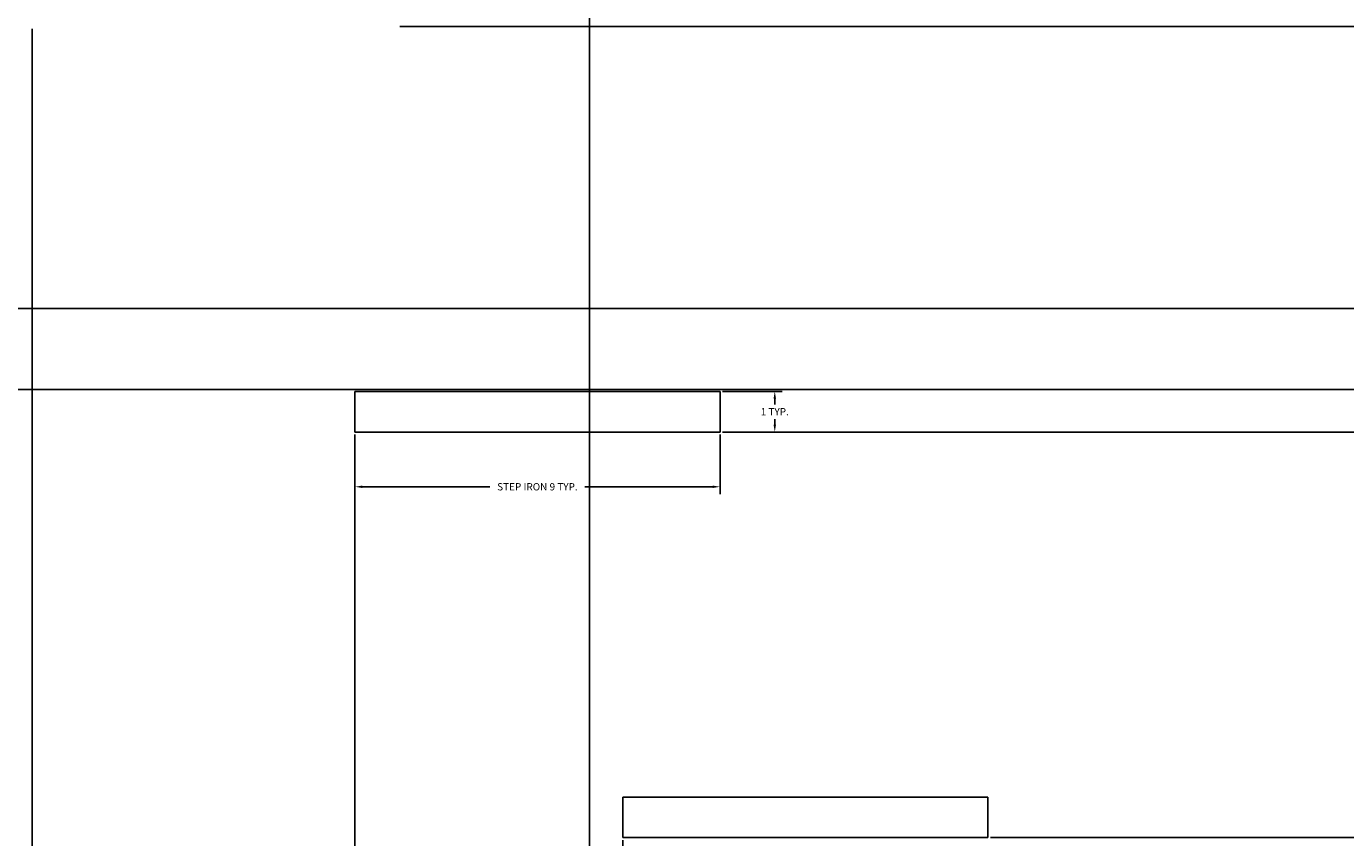
# Model space of a CAD drawing. Units: inches. Extents: x 2812 to 3051, y 1398 to 1659.
# Tile 17 of 65: x 2897 to 2929, y 1437 to 1457. Entities that reach past the tile are written whole.
import ezdxf

# ---------------------------------------------------------------- set-up
doc = ezdxf.new("R2010")
doc.units = ezdxf.units.IN
doc.layers.add('A-ANNO-DIMS', color=2, linetype='Continuous', lineweight=18)
doc.layers.add('S-STEP', color=3, linetype='Continuous', lineweight=25)
doc.styles.get("Standard").update_dxf_attribs({"font": 'arial.ttf'})
doc.dimstyles.get("Standard").update_dxf_attribs({"dimtxt": 0.18, "dimasz": 0.18, "dimexe": 0.18, "dimexo": 0.0625, "dimgap": 0.09, "dimtad": 0, "dimtih": 1, "dimtoh": 1, "dimdec": 4, "dimzin": 0, "dimdsep": 46, "dimtxsty": 'Standard', "dimcen": 0.09, "dimadec": 0, "dimazin": 0, "dimtfac": 1, "dimtdec": 4, "dimtofl": 0, "dimtmove": 0, "dimatfit": 3, "dimfxl": 1, "dimtolj": 1, "dimtzin": 0, "dimarcsym": 0})

# ---------------------------------------------------------------- blocks, each defined once
blk = doc.blocks.new('STEP-IRON-1')
for p, q in [((9, 1), (0, 1)), ((0, 1), (0, 0)), ((9, 0), (9, 1)), ((0, 0), (9, 0)), ((0, 0), (5.792, 0)), ((0, 0), (1.139, 0))]:
    blk.add_line(p, q)
blk = doc.blocks.new('STEP-IRON-2')
for p, q in [((9, 1), (0, 1)), ((0, 1), (0, 0)), ((9, 0), (9, 1)), ((0, 0), (3.641, 0)), ((0, 0), (9, 0)), ((0, 0), (5.792, 0))]:
    blk.add_line(p, q)
blk = doc.blocks.new('*D10')
at = {"layer": 'A-ANNO-DIMS', "color": 0, "lineweight": -2, "transparency": 16777216}
for p, q in [((2904.955, 1447.364), (2904.955, 1445.896)), ((2913.955, 1447.364), (2913.955, 1445.896)), ((2905.135, 1446.076), (2908.285, 1446.076)), ((2913.775, 1446.076), (2910.625, 1446.076))]:
    blk.add_line(p, q, dxfattribs=at)
at = {"layer": 'A-ANNO-DIMS', "color": 0, "transparency": 16777216}
for points in [[(2905.135, 1446.106), (2905.135, 1446.046), (2904.955, 1446.076)], [(2913.775, 1446.106), (2913.775, 1446.046), (2913.955, 1446.076)]]:
    blk.add_solid(points, dxfattribs=at)
at = {"layer": 'Defpoints', "color": 0, "transparency": 16777216}
for p in [(2904.955, 1447.426), (2913.955, 1447.426), (2913.955, 1446.076)]:
    blk.add_point(p, dxfattribs=at)
at = {"layer": 'A-ANNO-DIMS', "color": 0, "transparency": 16777216, "insert": (2909.455, 1446.076), "char_height": 0.18, "attachment_point": 5}
blk.add_mtext('\\A1;STEP IRON 9 TYP.', dxfattribs=at)
blk = doc.blocks.new('*D11')
at = {"layer": 'A-ANNO-DIMS', "color": 0, "lineweight": -2, "transparency": 16777216}
for p, q in [((2914.018, 1448.426), (2915.485, 1448.426)), ((2915.305, 1448.246), (2915.305, 1448.107)), ((2915.305, 1447.606), (2915.305, 1447.746)), ((2914.018, 1447.426), (2915.485, 1447.426))]:
    blk.add_line(p, q, dxfattribs=at)
at = {"layer": 'A-ANNO-DIMS', "color": 0, "transparency": 16777216}
for points in [[(2915.275, 1448.246), (2915.335, 1448.246), (2915.305, 1448.426)], [(2915.275, 1447.606), (2915.335, 1447.606), (2915.305, 1447.426)]]:
    blk.add_solid(points, dxfattribs=at)
at = {"layer": 'Defpoints', "color": 0, "transparency": 16777216}
for p in [(2913.955, 1448.426), (2915.305, 1448.426), (2913.955, 1447.426)]:
    blk.add_point(p, dxfattribs=at)
at = {"layer": 'A-ANNO-DIMS', "color": 0, "transparency": 16777216, "insert": (2915.305, 1447.926), "char_height": 0.18, "attachment_point": 5}
blk.add_mtext('\\A1;1 TYP.', dxfattribs=at)
blk = doc.blocks.new('*D29')
at = {"layer": 'A-ANNO-DIMS', "color": 0, "lineweight": -2, "transparency": 16777216}
for p, q in [((2910.742, 1598.757), (2910.742, 1397.505)), ((2883.385, 1559.757), (2883.385, 1397.505)), ((2883.565, 1397.685), (2896.598, 1397.685)), ((2910.562, 1397.685), (2897.528, 1397.685))]:
    blk.add_line(p, q, dxfattribs=at)
at = {"layer": 'A-ANNO-DIMS', "color": 0, "transparency": 16777216}
for points in [[(2883.565, 1397.715), (2883.565, 1397.655), (2883.385, 1397.685)], [(2910.562, 1397.715), (2910.562, 1397.655), (2910.742, 1397.685)]]:
    blk.add_solid(points, dxfattribs=at)
at = {"layer": 'Defpoints', "color": 0, "transparency": 16777216}
for p in [(2910.742, 1598.82), (2883.385, 1559.82), (2910.742, 1397.685)]:
    blk.add_point(p, dxfattribs=at)
at = {"layer": 'A-ANNO-DIMS', "color": 0, "transparency": 16777216, "insert": (2897.063, 1397.685), "char_height": 0.18, "attachment_point": 5}
blk.add_mtext('\\A1;27.357', dxfattribs=at)
blk = doc.blocks.new('*D45')
at = {"layer": 'A-ANNO-DIMS', "color": 0, "lineweight": -2, "transparency": 16777216}
for p, q in [((2896.385, 1487.973), (2896.385, 1397.505)), ((2941.385, 1487.973), (2941.385, 1397.505)), ((2896.565, 1397.685), (2918.662, 1397.685)), ((2941.205, 1397.685), (2919.108, 1397.685))]:
    blk.add_line(p, q, dxfattribs=at)
at = {"layer": 'A-ANNO-DIMS', "color": 0, "transparency": 16777216}
for points in [[(2896.565, 1397.715), (2896.565, 1397.655), (2896.385, 1397.685)], [(2941.205, 1397.715), (2941.205, 1397.655), (2941.385, 1397.685)]]:
    blk.add_solid(points, dxfattribs=at)
at = {"layer": 'Defpoints', "color": 0, "transparency": 16777216}
for p in [(2896.385, 1488.035), (2941.385, 1488.035), (2941.385, 1397.685)]:
    blk.add_point(p, dxfattribs=at)
at = {"layer": 'A-ANNO-DIMS', "color": 0, "transparency": 16777216, "insert": (2918.885, 1397.685), "char_height": 0.18, "attachment_point": 5}
blk.add_mtext('\\A1;45', dxfattribs=at)
blk = doc.blocks.new('*D56')
at = {"layer": 'A-ANNO-DIMS', "color": 0, "lineweight": -2, "transparency": 16777216}
for p, q in [((2880.322, 1452.035), (2811.806, 1452.035)), ((2811.986, 1451.855), (2811.986, 1434.217)), ((2811.986, 1416.215), (2811.986, 1433.853)), ((2952.322, 1416.035), (2811.806, 1416.035))]:
    blk.add_line(p, q, dxfattribs=at)
at = {"layer": 'A-ANNO-DIMS', "color": 0, "transparency": 16777216}
for points in [[(2811.956, 1451.855), (2812.016, 1451.855), (2811.986, 1452.035)], [(2811.956, 1416.215), (2812.016, 1416.215), (2811.986, 1416.035)]]:
    blk.add_solid(points, dxfattribs=at)
at = {"layer": 'Defpoints', "color": 0, "transparency": 16777216}
for p in [(2811.986, 1452.035), (2880.385, 1452.035), (2952.385, 1416.035)]:
    blk.add_point(p, dxfattribs=at)
at = {"layer": 'A-ANNO-DIMS', "color": 0, "transparency": 16777216, "insert": (2811.986, 1434.035), "char_height": 0.18, "attachment_point": 5}
blk.add_mtext('\\A1;36', dxfattribs=at)
blk = doc.blocks.new('*D60')
at = {"layer": 'A-ANNO-DIMS', "color": 0, "lineweight": -2, "transparency": 16777216}
for p, q in [((2889.058, 1466.34), (2889.058, 1397.505)), ((2897.002, 1457.364), (2897.002, 1397.505)), ((2889.238, 1397.685), (2892.637, 1397.685)), ((2896.822, 1397.685), (2893.422, 1397.685))]:
    blk.add_line(p, q, dxfattribs=at)
at = {"layer": 'A-ANNO-DIMS', "color": 0, "transparency": 16777216}
for points in [[(2889.238, 1397.715), (2889.238, 1397.655), (2889.058, 1397.685)], [(2896.822, 1397.715), (2896.822, 1397.655), (2897.002, 1397.685)]]:
    blk.add_solid(points, dxfattribs=at)
at = {"layer": 'Defpoints', "color": 0, "transparency": 16777216}
for p in [(2889.058, 1466.402), (2897.002, 1457.426), (2897.002, 1397.685)]:
    blk.add_point(p, dxfattribs=at)
at = {"layer": 'A-ANNO-DIMS', "color": 0, "transparency": 16777216, "insert": (2893.03, 1397.685), "char_height": 0.18, "attachment_point": 5}
blk.add_mtext('\\A1;7.944', dxfattribs=at)
blk = doc.blocks.new('*D61')
at = {"layer": 'A-ANNO-DIMS', "color": 0, "lineweight": -2, "transparency": 16777216}
for p, q in [((2897.002, 1457.364), (2897.002, 1397.505)), ((2904.955, 1447.364), (2904.955, 1397.505)), ((2897.182, 1397.685), (2900.586, 1397.685)), ((2904.775, 1397.685), (2901.372, 1397.685))]:
    blk.add_line(p, q, dxfattribs=at)
at = {"layer": 'A-ANNO-DIMS', "color": 0, "transparency": 16777216}
for points in [[(2897.182, 1397.715), (2897.182, 1397.655), (2897.002, 1397.685)], [(2904.775, 1397.715), (2904.775, 1397.655), (2904.955, 1397.685)]]:
    blk.add_solid(points, dxfattribs=at)
at = {"layer": 'Defpoints', "color": 0, "transparency": 16777216}
for p in [(2897.002, 1457.426), (2904.955, 1447.426), (2904.955, 1397.685)]:
    blk.add_point(p, dxfattribs=at)
at = {"layer": 'A-ANNO-DIMS', "color": 0, "transparency": 16777216, "insert": (2900.979, 1397.685), "char_height": 0.18, "attachment_point": 5}
blk.add_mtext('\\A1;7.953', dxfattribs=at)
blk = doc.blocks.new('*D62')
at = {"layer": 'A-ANNO-DIMS', "color": 0, "lineweight": -2, "transparency": 16777216}
for p, q in [((2904.955, 1447.364), (2904.955, 1397.505)), ((2911.558, 1437.364), (2911.558, 1397.505)), ((2905.135, 1397.685), (2907.862, 1397.685)), ((2911.378, 1397.685), (2908.651, 1397.685))]:
    blk.add_line(p, q, dxfattribs=at)
at = {"layer": 'A-ANNO-DIMS', "color": 0, "transparency": 16777216}
for points in [[(2905.135, 1397.715), (2905.135, 1397.655), (2904.955, 1397.685)], [(2911.378, 1397.715), (2911.378, 1397.655), (2911.558, 1397.685)]]:
    blk.add_solid(points, dxfattribs=at)
at = {"layer": 'Defpoints', "color": 0, "transparency": 16777216}
for p in [(2904.955, 1447.426), (2911.558, 1437.426), (2911.558, 1397.685)]:
    blk.add_point(p, dxfattribs=at)
at = {"layer": 'A-ANNO-DIMS', "color": 0, "transparency": 16777216, "insert": (2908.256, 1397.685), "char_height": 0.18, "attachment_point": 5}
blk.add_mtext('\\A1;6.603', dxfattribs=at)
blk = doc.blocks.new('*D66')
at = {"layer": 'A-ANNO-DIMS', "color": 0, "lineweight": -2, "transparency": 16777216}
for p, q in [((2914.018, 1447.426), (3051.178, 1447.426)), ((3050.998, 1447.246), (3050.998, 1442.608)), ((3050.998, 1437.606), (3050.998, 1442.245)), ((2920.62, 1437.426), (3051.178, 1437.426))]:
    blk.add_line(p, q, dxfattribs=at)
at = {"layer": 'A-ANNO-DIMS', "color": 0, "transparency": 16777216}
for points in [[(3050.968, 1447.246), (3051.028, 1447.246), (3050.998, 1447.426)], [(3050.968, 1437.606), (3051.028, 1437.606), (3050.998, 1437.426)]]:
    blk.add_solid(points, dxfattribs=at)
at = {"layer": 'Defpoints', "color": 0, "transparency": 16777216}
for p in [(2913.955, 1447.426), (3050.998, 1447.426), (2920.558, 1437.426)]:
    blk.add_point(p, dxfattribs=at)
at = {"layer": 'A-ANNO-DIMS', "color": 0, "transparency": 16777216, "insert": (3050.998, 1442.426), "char_height": 0.18, "attachment_point": 5}
blk.add_mtext('\\A1;10', dxfattribs=at)
blk = doc.blocks.new('*D67')
at = {"layer": 'A-ANNO-DIMS', "color": 0, "lineweight": -2, "transparency": 16777216}
for p, q in [((2906.065, 1457.426), (3051.178, 1457.426)), ((3050.998, 1457.246), (3050.998, 1452.608)), ((3050.998, 1447.606), (3050.998, 1452.245)), ((2914.018, 1447.426), (3051.178, 1447.426))]:
    blk.add_line(p, q, dxfattribs=at)
at = {"layer": 'A-ANNO-DIMS', "color": 0, "transparency": 16777216}
for points in [[(3050.968, 1457.246), (3051.028, 1457.246), (3050.998, 1457.426)], [(3050.968, 1447.606), (3051.028, 1447.606), (3050.998, 1447.426)]]:
    blk.add_solid(points, dxfattribs=at)
at = {"layer": 'Defpoints', "color": 0, "transparency": 16777216}
for p in [(2906.002, 1457.426), (3050.998, 1457.426), (2913.955, 1447.426)]:
    blk.add_point(p, dxfattribs=at)
at = {"layer": 'A-ANNO-DIMS', "color": 0, "transparency": 16777216, "insert": (3050.998, 1452.426), "char_height": 0.18, "attachment_point": 5}
blk.add_mtext('\\A1;10', dxfattribs=at)
blk = doc.blocks.new('*D68')
at = {"layer": 'A-ANNO-DIMS', "color": 0, "lineweight": -2, "transparency": 16777216}
for p, q in [((2898.12, 1466.402), (3051.178, 1466.402)), ((3050.998, 1466.222), (3050.998, 1462.096)), ((3050.998, 1457.606), (3050.998, 1461.733)), ((2906.065, 1457.426), (3051.178, 1457.426))]:
    blk.add_line(p, q, dxfattribs=at)
at = {"layer": 'A-ANNO-DIMS', "color": 0, "transparency": 16777216}
for points in [[(3050.968, 1466.222), (3051.028, 1466.222), (3050.998, 1466.402)], [(3050.968, 1457.606), (3051.028, 1457.606), (3050.998, 1457.426)]]:
    blk.add_solid(points, dxfattribs=at)
at = {"layer": 'Defpoints', "color": 0, "transparency": 16777216}
for p in [(2898.058, 1466.402), (3050.998, 1466.402), (2906.002, 1457.426)]:
    blk.add_point(p, dxfattribs=at)
at = {"layer": 'A-ANNO-DIMS', "color": 0, "transparency": 16777216, "insert": (3050.998, 1461.914), "char_height": 0.18, "attachment_point": 5}
blk.add_mtext('\\A1;8.976', dxfattribs=at)
blk = doc.blocks.new('*D75')
at = {"layer": 'A-ANNO-DIMS', "color": 0, "lineweight": -2, "transparency": 16777216}
for p, q in [((2963.812, 1448.474), (2811.806, 1448.474)), ((2811.986, 1448.294), (2811.986, 1432.437)), ((2811.986, 1416.215), (2811.986, 1432.073)), ((2961.322, 1416.035), (2811.806, 1416.035))]:
    blk.add_line(p, q, dxfattribs=at)
at = {"layer": 'A-ANNO-DIMS', "color": 0, "transparency": 16777216}
for points in [[(2811.956, 1448.294), (2812.016, 1448.294), (2811.986, 1448.474)], [(2811.956, 1416.215), (2812.016, 1416.215), (2811.986, 1416.035)]]:
    blk.add_solid(points, dxfattribs=at)
at = {"layer": 'Defpoints', "color": 0, "transparency": 16777216}
for p in [(2811.986, 1448.474), (2963.874, 1448.474), (2961.385, 1416.035)]:
    blk.add_point(p, dxfattribs=at)
at = {"layer": 'A-ANNO-DIMS', "color": 0, "transparency": 16777216, "insert": (2811.986, 1432.255), "char_height": 0.18, "attachment_point": 5}
blk.add_mtext('\\A1;32.44', dxfattribs=at)
blk = doc.blocks.new('*D76')
at = {"layer": 'A-ANNO-DIMS', "color": 0, "lineweight": -2, "transparency": 16777216}
for p, q in [((2963.812, 1450.474), (2811.806, 1450.474)), ((2811.986, 1450.294), (2811.986, 1449.654)), ((2811.986, 1448.654), (2811.986, 1449.293)), ((2963.812, 1448.474), (2811.806, 1448.474))]:
    blk.add_line(p, q, dxfattribs=at)
at = {"layer": 'A-ANNO-DIMS', "color": 0, "transparency": 16777216}
for points in [[(2811.956, 1450.294), (2812.016, 1450.294), (2811.986, 1450.474)], [(2811.956, 1448.654), (2812.016, 1448.654), (2811.986, 1448.474)]]:
    blk.add_solid(points, dxfattribs=at)
at = {"layer": 'Defpoints', "color": 0, "transparency": 16777216}
for p in [(2811.986, 1450.474), (2963.874, 1450.474), (2963.874, 1448.474)]:
    blk.add_point(p, dxfattribs=at)
at = {"layer": 'A-ANNO-DIMS', "color": 0, "transparency": 16777216, "insert": (2811.986, 1449.474), "char_height": 0.18, "attachment_point": 5}
blk.add_mtext('\\A1;2', dxfattribs=at)
blk = doc.blocks.new('*D77')
at = {"layer": 'A-ANNO-DIMS', "color": 0, "lineweight": -2, "transparency": 16777216}
for p, q in [((2961.322, 1472.035), (2811.806, 1472.035)), ((2811.986, 1471.855), (2811.986, 1461.436)), ((2811.986, 1450.654), (2811.986, 1461.073)), ((2963.812, 1450.474), (2811.806, 1450.474))]:
    blk.add_line(p, q, dxfattribs=at)
at = {"layer": 'A-ANNO-DIMS', "color": 0, "transparency": 16777216}
for points in [[(2811.956, 1471.855), (2812.016, 1471.855), (2811.986, 1472.035)], [(2811.956, 1450.654), (2812.016, 1450.654), (2811.986, 1450.474)]]:
    blk.add_solid(points, dxfattribs=at)
at = {"layer": 'Defpoints', "color": 0, "transparency": 16777216}
for p in [(2811.986, 1472.035), (2961.385, 1472.035), (2963.874, 1450.474)]:
    blk.add_point(p, dxfattribs=at)
at = {"layer": 'A-ANNO-DIMS', "color": 0, "transparency": 16777216, "insert": (2811.986, 1461.255), "char_height": 0.18, "attachment_point": 5}
blk.add_mtext('\\A1;21.56', dxfattribs=at)

msp = doc.modelspace()

# ---------------------------------------------------------------- block references
at = {"layer": 'S-STEP'}
for name, p in [('STEP-IRON-1', (2904.9553, 1447.4261)), ('STEP-IRON-2', (2911.5574, 1437.4261))]:
    msp.add_blockref(name, p, dxfattribs=at)

# ---------------------------------------------------------------- dimensions: what is measured, and where the dimension line sits
at = {"layer": 'A-ANNO-DIMS'}
for base, p1, p2, override, picture, middle in [((2910.7415, 1397.6854), (2883.3849, 1559.82), (2910.7415, 1598.82), {"dimdec": 3, "dimlfac": 1, "dimrnd": 0, "dimzin": 0, "dimdsep": 46, "dimlunit": 2}, '*D29', (2897.0632, 1397.6854)), ((2941.3849, 1397.6854), (2896.3849, 1488.0354), (2941.3849, 1488.0354), {"dimdec": 0, "dimlfac": 1, "dimrnd": 0, "dimzin": 0, "dimdsep": 46, "dimlunit": 2}, '*D45', (2918.8849, 1397.6854)), ((2897.0021, 1397.6854), (2889.0577, 1466.4024), (2897.0021, 1457.4265), {"dimdec": 3, "dimlfac": 1, "dimrnd": 0, "dimzin": 0, "dimdsep": 46, "dimlunit": 2}, '*D60', (2893.0299, 1397.6854)), ((2904.9551, 1397.6854), (2897.0021, 1457.4265), (2904.9551, 1447.4265), {"dimdec": 3, "dimlfac": 1, "dimrnd": 0, "dimzin": 0, "dimdsep": 46, "dimlunit": 2}, '*D61', (2900.9786, 1397.6854)), ((2911.5577, 1397.6854), (2904.9551, 1447.4265), (2911.5577, 1437.4265), {"dimdec": 3, "dimlfac": 1, "dimrnd": 0, "dimzin": 0, "dimdsep": 46, "dimlunit": 2}, '*D62', (2908.2564, 1397.6854))]:
    dim = msp.add_linear_dim(base=base, p1=p1, p2=p2, dimstyle='Standard', override=override, dxfattribs=at)
    dim.commit()
    dim.dimension.update_dxf_attribs({"geometry": picture, "text_midpoint": middle})
for base, p1, p2, override, picture, middle in [((2811.9855, 1472.0354), (2963.8741, 1450.4738), (2961.3849, 1472.0354), {"dimdec": 2, "dimlfac": 1, "dimrnd": 0, "dimzin": 0, "dimdsep": 46, "dimlunit": 2}, '*D77', (2811.9855, 1461.2546)), ((3050.998, 1466.4024), (2906.0021, 1457.4265), (2898.0577, 1466.4024), {"dimdec": 3, "dimlfac": 1, "dimrnd": 0, "dimzin": 0, "dimdsep": 46, "dimlunit": 2}, '*D68', (3050.998, 1461.9144)), ((3050.998, 1457.4265), (2913.9551, 1447.4265), (2906.0021, 1457.4265), {"dimdec": 0, "dimlfac": 1, "dimrnd": 0, "dimzin": 0, "dimdsep": 46, "dimlunit": 2}, '*D67', (3050.998, 1452.4265)), ((2811.9855, 1452.0354), (2952.3849, 1416.0354), (2880.3849, 1452.0354), {"dimdec": 0, "dimlfac": 1, "dimrnd": 0, "dimzin": 0, "dimdsep": 46, "dimlunit": 2}, '*D56', (2811.9855, 1434.0354)), ((2811.9855, 1450.4738), (2963.8741, 1448.4738), (2963.8741, 1450.4738), {"dimdec": 0, "dimlfac": 1, "dimrnd": 0, "dimzin": 0, "dimdsep": 46, "dimlunit": 2}, '*D76', (2811.9855, 1449.4738)), ((2811.9855, 1448.4738), (2961.3849, 1416.0354), (2963.8741, 1448.4738), {"dimdec": 2, "dimlfac": 1, "dimrnd": 0, "dimzin": 0, "dimdsep": 46, "dimlunit": 2}, '*D75', (2811.9855, 1432.2546)), ((3050.998, 1447.4265), (2920.5577, 1437.4265), (2913.9551, 1447.4265), {"dimdec": 0, "dimlfac": 1, "dimrnd": 0, "dimzin": 0, "dimdsep": 46, "dimlunit": 2}, '*D66', (3050.998, 1442.4265))]:
    dim = msp.add_linear_dim(base=base, p1=p1, p2=p2, angle=90, dimstyle='Standard', override=override, dxfattribs=at)
    dim.commit()
    dim.dimension.update_dxf_attribs({"geometry": picture, "text_midpoint": middle})
dim = msp.add_linear_dim(base=(2915.3051, 1448.4265), p1=(2913.9551, 1447.4265), p2=(2913.9551, 1448.4265), angle=90, text='<> TYP.', dimstyle='Standard', override={"dimdec": 0, "dimlfac": 1, "dimrnd": 0, "dimzin": 0, "dimdsep": 46, "dimlunit": 2}, dxfattribs=at)
dim.commit()
dim.dimension.update_dxf_attribs({"geometry": '*D11', "text_midpoint": (2915.3051, 1447.9265)})
dim = msp.add_linear_dim(base=(2913.9551, 1446.0765), p1=(2904.9551, 1447.4265), p2=(2913.9551, 1447.4265), text='STEP IRON <> TYP.', dimstyle='Standard', override={"dimdec": 0, "dimlfac": 1, "dimrnd": 0, "dimzin": 0, "dimdsep": 46, "dimlunit": 2}, dxfattribs=at)
dim.commit()
dim.dimension.update_dxf_attribs({"geometry": '*D10', "text_midpoint": (2909.4551, 1446.0765)})

doc.saveas('drawing.dxf')
